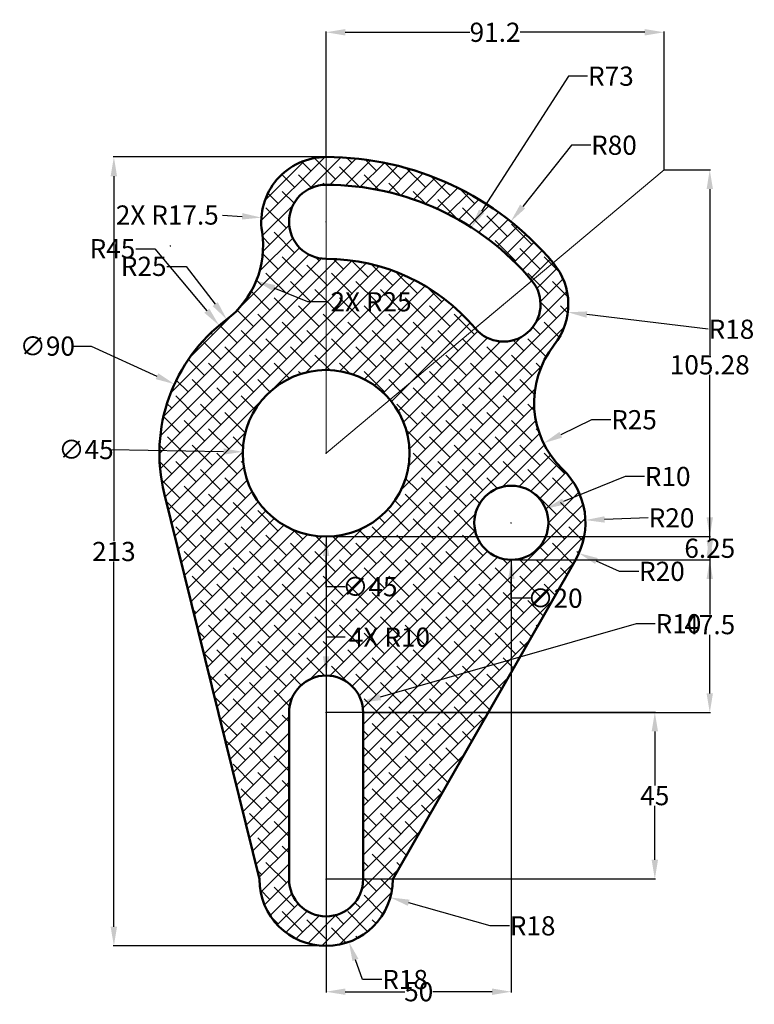
# Model space of a CAD drawing. Units: millimetres. Extents: x 3 to 201, y -134 to 131.
import ezdxf

# ---------------------------------------------------------------- set-up
doc = ezdxf.new("R2010")
doc.units = ezdxf.units.MM
doc.header["$MEASUREMENT"] = 0
for name, color, linetype, lineweight in [('M-CONS', 51, 'Continuous', 13), ('M-DIMS', 85, 'Continuous', 25), ('M-HATC', 241, 'Continuous', 18), ('M-OUTL', 11, 'Continuous', 50)]:
    doc.layers.add(name, color=color, linetype=linetype, lineweight=lineweight)
doc.styles.get("Standard").update_dxf_attribs({"font": 'arial.ttf'})
doc.dimstyles.get("Standard").update_dxf_attribs({"dimtxt": 5.18, "dimasz": 5.18, "dimexe": 0.18, "dimexo": 0.0625, "dimgap": 0.09, "dimtad": 0, "dimtih": 1, "dimtoh": 1, "dimdec": 0, "dimzin": 0, "dimdsep": 46, "dimtxsty": 'Standard', "dimcen": 0.09, "dimadec": 0, "dimazin": 0, "dimtfac": 1, "dimtdec": 0, "dimtofl": 0, "dimtmove": 0, "dimatfit": 3, "dimfxl": 1, "dimtolj": 1, "dimtzin": 0, "dimarcsym": 0})

# ---------------------------------------------------------------- blocks, each defined once
blk = doc.blocks.new('*D1')
at = {"layer": 'Defpoints', "color": 0, "transparency": 16777216}
for p in [(133.74, 54.52), (151.12, 52.43)]:
    blk.add_point(p, dxfattribs=at)
at = {"layer": 'M-DIMS', "color": 0, "lineweight": -2, "transparency": 16777216}
for p, q in [((133.65, 54.52), (133.83, 54.52)), ((133.74, 54.43), (133.74, 54.61)), ((188.99, 47.85), (156.26, 51.8))]:
    blk.add_line(p, q, dxfattribs=at)
at = {"layer": 'M-DIMS', "color": 0, "transparency": 16777216}
blk.add_solid([(156.36, 52.66), (156.15, 50.95), (151.12, 52.43)], dxfattribs=at)
at = {"layer": 'M-DIMS', "color": 0, "transparency": 16777216, "insert": (195.27, 47.85), "char_height": 5.18, "attachment_point": 5}
blk.add_mtext('\\A1;R18', dxfattribs=at)
blk = doc.blocks.new('*D2')
at = {"layer": 'Defpoints', "color": 0, "transparency": 16777216}
for p in [(135.7, 76.93), (85.86, 14.35)]:
    blk.add_point(p, dxfattribs=at)
at = {"layer": 'M-DIMS', "color": 0, "lineweight": -2, "transparency": 16777216}
for p, q in [((152.11, 97.53), (138.93, 80.98)), ((157.29, 97.53), (152.11, 97.53)), ((85.77, 14.35), (85.95, 14.35)), ((85.86, 14.26), (85.86, 14.44))]:
    blk.add_line(p, q, dxfattribs=at)
at = {"layer": 'M-DIMS', "color": 0, "transparency": 16777216}
blk.add_solid([(138.25, 81.52), (139.6, 80.44), (135.7, 76.93)], dxfattribs=at)
at = {"layer": 'M-DIMS', "color": 0, "transparency": 16777216, "insert": (163.56, 97.53), "char_height": 5.18, "attachment_point": 5}
blk.add_mtext('\\A1;R80', dxfattribs=at)
blk = doc.blocks.new('*D3')
at = {"layer": 'Defpoints', "color": 0, "transparency": 16777216}
for p in [(125.05, 75.35), (85.86, 14.35)]:
    blk.add_point(p, dxfattribs=at)
at = {"layer": 'M-DIMS', "color": 0, "lineweight": -2, "transparency": 16777216}
for p, q in [((151.28, 116.17), (127.85, 79.7)), ((156.46, 116.17), (151.28, 116.17)), ((85.77, 14.35), (85.95, 14.35)), ((85.86, 14.26), (85.86, 14.44))]:
    blk.add_line(p, q, dxfattribs=at)
at = {"layer": 'M-DIMS', "color": 0, "transparency": 16777216}
blk.add_solid([(127.13, 80.17), (128.58, 79.24), (125.05, 75.35)], dxfattribs=at)
at = {"layer": 'M-DIMS', "color": 0, "transparency": 16777216, "insert": (162.74, 116.17), "char_height": 5.18, "attachment_point": 5}
blk.add_mtext('\\A1;R73', dxfattribs=at)
blk = doc.blocks.new('*D4')
at = {"layer": 'Defpoints', "color": 0, "transparency": 16777216}
for p in [(167.01, 28.08), (144.56, 17.09)]:
    blk.add_point(p, dxfattribs=at)
at = {"layer": 'M-DIMS', "color": 0, "lineweight": -2, "transparency": 16777216}
for p, q in [((157.5, 23.42), (149.21, 19.36)), ((162.68, 23.42), (157.5, 23.42))]:
    blk.add_line(p, q, dxfattribs=at)
at = {"layer": 'M-DIMS', "color": 0, "transparency": 16777216}
blk.add_solid([(148.83, 20.14), (149.59, 18.59), (144.56, 17.09)], dxfattribs=at)
at = {"layer": 'M-DIMS', "color": 0, "transparency": 16777216, "insert": (168.98, 23.42), "char_height": 5.18, "attachment_point": 5}
blk.add_mtext('\\A1;R25', dxfattribs=at)
blk = doc.blocks.new('*D5')
at = {"layer": 'Defpoints', "color": 0, "transparency": 16777216}
for p in [(135.86, -4.4), (155.85, -3.68)]:
    blk.add_point(p, dxfattribs=at)
at = {"layer": 'M-DIMS', "color": 0, "lineweight": -2, "transparency": 16777216}
for p, q in [((135.77, -4.4), (135.95, -4.4)), ((135.86, -4.49), (135.86, -4.31)), ((172.83, -3.08), (161.03, -3.5))]:
    blk.add_line(p, q, dxfattribs=at)
at = {"layer": 'M-DIMS', "color": 0, "transparency": 16777216}
blk.add_solid([(161, -2.64), (161.06, -4.36), (155.85, -3.68)], dxfattribs=at)
at = {"layer": 'M-DIMS', "color": 0, "transparency": 16777216, "insert": (179.1, -3.08), "char_height": 5.18, "attachment_point": 5}
blk.add_mtext('\\A1;R20', dxfattribs=at)
blk = doc.blocks.new('*D6')
at = {"layer": 'Defpoints', "color": 0, "transparency": 16777216}
for p in [(145.13, -0.63), (135.86, -4.4)]:
    blk.add_point(p, dxfattribs=at)
at = {"layer": 'M-DIMS', "color": 0, "lineweight": -2, "transparency": 16777216}
for p, q in [((166.61, 8.1), (149.93, 1.32)), ((171.79, 8.1), (166.61, 8.1)), ((135.77, -4.4), (135.95, -4.4)), ((135.86, -4.49), (135.86, -4.31))]:
    blk.add_line(p, q, dxfattribs=at)
at = {"layer": 'M-DIMS', "color": 0, "transparency": 16777216}
blk.add_solid([(149.6, 2.12), (150.25, 0.52), (145.13, -0.63)], dxfattribs=at)
at = {"layer": 'M-DIMS', "color": 0, "transparency": 16777216, "insert": (178.06, 8.1), "char_height": 5.18, "attachment_point": 5}
blk.add_mtext('\\A1;R10', dxfattribs=at)
blk = doc.blocks.new('*D7')
at = {"layer": 'Defpoints', "color": 0, "transparency": 16777216}
for p in [(95.48, -52.89), (85.86, -55.65)]:
    blk.add_point(p, dxfattribs=at)
at = {"layer": 'M-DIMS', "color": 0, "lineweight": -2, "transparency": 16777216}
for p, q in [((169.51, -31.65), (100.45, -51.46)), ((174.69, -31.65), (169.51, -31.65)), ((85.77, -55.65), (85.95, -55.65)), ((85.86, -55.74), (85.86, -55.56))]:
    blk.add_line(p, q, dxfattribs=at)
at = {"layer": 'M-DIMS', "color": 0, "transparency": 16777216}
blk.add_solid([(100.22, -50.63), (100.69, -52.29), (95.48, -52.89)], dxfattribs=at)
at = {"layer": 'M-DIMS', "color": 0, "transparency": 16777216, "insert": (180.96, -31.65), "char_height": 5.18, "attachment_point": 5}
blk.add_mtext('\\A1;R10', dxfattribs=at)
blk = doc.blocks.new('*D8')
at = {"layer": 'Defpoints', "color": 0, "transparency": 16777216}
for p in [(85.86, -100.65), (103.18, -105.56)]:
    blk.add_point(p, dxfattribs=at)
at = {"layer": 'M-DIMS', "color": 0, "lineweight": -2, "transparency": 16777216}
for p, q in [((85.77, -100.65), (85.95, -100.65)), ((85.86, -100.74), (85.86, -100.56)), ((130.15, -113.21), (108.16, -106.98)), ((135.33, -113.21), (130.15, -113.21))]:
    blk.add_line(p, q, dxfattribs=at)
at = {"layer": 'M-DIMS', "color": 0, "transparency": 16777216}
blk.add_solid([(108.4, -106.15), (107.93, -107.81), (103.18, -105.56)], dxfattribs=at)
at = {"layer": 'M-DIMS', "color": 0, "transparency": 16777216, "insert": (141.61, -113.21), "char_height": 5.18, "attachment_point": 5}
blk.add_mtext('\\A1;R18', dxfattribs=at)
blk = doc.blocks.new('*D9')
at = {"layer": 'Defpoints', "color": 0, "transparency": 16777216}
for p in [(43.86, 70.35), (59.07, 50.51)]:
    blk.add_point(p, dxfattribs=at)
at = {"layer": 'M-DIMS', "color": 0, "lineweight": -2, "transparency": 16777216}
for p, q in [((42.92, 64.83), (48.1, 64.83)), ((48.1, 64.83), (55.92, 54.62))]:
    blk.add_line(p, q, dxfattribs=at)
at = {"layer": 'M-DIMS', "color": 0, "transparency": 16777216}
blk.add_solid([(56.61, 55.15), (55.24, 54.1), (59.07, 50.51)], dxfattribs=at)
at = {"layer": 'M-DIMS', "color": 0, "transparency": 16777216, "insert": (36.62, 64.83), "char_height": 5.18, "attachment_point": 5}
blk.add_mtext('\\A1;R25', dxfattribs=at)
blk = doc.blocks.new('*D10')
at = {"layer": 'Defpoints', "color": 0, "transparency": 16777216}
for p in [(44.92, 33.03), (126.81, -4.33)]:
    blk.add_point(p, dxfattribs=at)
at = {"layer": 'M-DIMS', "color": 0, "lineweight": -2, "transparency": 16777216}
for p, q in [((17.23, 43.3), (22.41, 43.3)), ((22.41, 43.3), (40.21, 35.18)), ((85.77, 14.35), (85.95, 14.35)), ((85.86, 14.26), (85.86, 14.44))]:
    blk.add_line(p, q, dxfattribs=at)
at = {"layer": 'M-DIMS', "color": 0, "transparency": 16777216}
blk.add_solid([(40.57, 35.96), (39.85, 34.39), (44.92, 33.03)], dxfattribs=at)
at = {"layer": 'M-DIMS', "color": 0, "transparency": 16777216, "insert": (10.62, 43.3), "char_height": 5.18, "attachment_point": 5}
blk.add_mtext('\\A1;∅90', dxfattribs=at)
blk = doc.blocks.new('*D11')
at = {"layer": 'Defpoints', "color": 0, "transparency": 16777216}
for p in [(63.37, 14.75), (108.36, 13.95)]:
    blk.add_point(p, dxfattribs=at)
at = {"layer": 'M-DIMS', "color": 0, "lineweight": -2, "transparency": 16777216}
for p, q in [((27.7, 15.38), (58.19, 14.84)), ((85.77, 14.35), (85.95, 14.35)), ((85.86, 14.26), (85.86, 14.44))]:
    blk.add_line(p, q, dxfattribs=at)
at = {"layer": 'M-DIMS', "color": 0, "transparency": 16777216}
blk.add_solid([(58.2, 15.7), (58.17, 13.98), (63.37, 14.75)], dxfattribs=at)
at = {"layer": 'M-DIMS', "color": 0, "transparency": 16777216, "insert": (21.06, 15.38), "char_height": 5.18, "attachment_point": 5}
blk.add_mtext('\\A1;∅45', dxfattribs=at)
blk = doc.blocks.new('*D12')
at = {"layer": 'Defpoints', "color": 0, "transparency": 16777216}
for p in [(85.86, -55.56), (85.86, -100.56), (174.59, -100.56)]:
    blk.add_point(p, dxfattribs=at)
at = {"layer": 'M-DIMS', "color": 0, "lineweight": -2, "transparency": 16777216}
for p, q in [((85.93, -55.56), (174.77, -55.56)), ((174.59, -60.74), (174.59, -75.34)), ((174.59, -95.38), (174.59, -80.78)), ((85.93, -100.56), (174.77, -100.56))]:
    blk.add_line(p, q, dxfattribs=at)
at = {"layer": 'M-DIMS', "color": 0, "transparency": 16777216}
for points in [[(173.73, -60.74), (175.45, -60.74), (174.59, -55.56)], [(173.73, -95.38), (175.45, -95.38), (174.59, -100.56)]]:
    blk.add_solid(points, dxfattribs=at)
at = {"layer": 'M-DIMS', "color": 0, "transparency": 16777216, "insert": (174.59, -78.06), "char_height": 5.18, "attachment_point": 5}
blk.add_mtext('\\A1;45', dxfattribs=at)
blk = doc.blocks.new('*D13')
at = {"layer": 'Defpoints', "color": 0, "transparency": 16777216}
for p in [(28.58, 94.35), (85.86, 94.35), (85.86, -118.65)]:
    blk.add_point(p, dxfattribs=at)
at = {"layer": 'M-DIMS', "color": 0, "lineweight": -2, "transparency": 16777216}
for p, q in [((85.8, 94.35), (28.4, 94.35)), ((28.58, 89.17), (28.58, -9.41)), ((28.58, -113.47), (28.58, -14.89)), ((85.8, -118.65), (28.4, -118.65))]:
    blk.add_line(p, q, dxfattribs=at)
at = {"layer": 'M-DIMS', "color": 0, "transparency": 16777216}
for points in [[(27.71, 89.17), (29.44, 89.17), (28.58, 94.35)], [(27.71, -113.47), (29.44, -113.47), (28.58, -118.65)]]:
    blk.add_solid(points, dxfattribs=at)
at = {"layer": 'M-DIMS', "color": 0, "transparency": 16777216, "insert": (28.58, -12.15), "char_height": 5.18, "attachment_point": 5}
blk.add_mtext('\\A1;213', dxfattribs=at)
blk = doc.blocks.new('*D14')
at = {"layer": 'Defpoints', "color": 0, "transparency": 16777216}
for p in [(85.86, -8.15), (189.42, -8.15), (95.86, -55.65)]:
    blk.add_point(p, dxfattribs=at)
at = {"layer": 'M-DIMS', "color": 0, "lineweight": -2, "transparency": 16777216}
for p, q in [((85.93, -8.15), (189.6, -8.15)), ((189.42, -13.33), (189.42, -29.18)), ((189.42, -50.47), (189.42, -34.62)), ((95.93, -55.65), (189.6, -55.65))]:
    blk.add_line(p, q, dxfattribs=at)
at = {"layer": 'M-DIMS', "color": 0, "transparency": 16777216}
for points in [[(188.56, -13.33), (190.28, -13.33), (189.42, -8.15)], [(188.56, -50.47), (190.28, -50.47), (189.42, -55.65)]]:
    blk.add_solid(points, dxfattribs=at)
at = {"layer": 'M-DIMS', "color": 0, "transparency": 16777216, "insert": (189.42, -31.9), "char_height": 5.18, "attachment_point": 5}
blk.add_mtext('\\A1;47.5', dxfattribs=at)
blk = doc.blocks.new('*D15')
at = {"layer": 'Defpoints', "color": 0, "transparency": 16777216}
for p in [(85.86, -8.15), (135.86, -14.4), (85.86, -131)]:
    blk.add_point(p, dxfattribs=at)
at = {"layer": 'M-DIMS', "color": 0, "lineweight": -2, "transparency": 16777216}
for p, q in [((85.86, -8.21), (85.86, -131.18)), ((135.86, -14.46), (135.86, -131.18)), ((91.04, -131), (107.07, -131)), ((130.68, -131), (114.65, -131))]:
    blk.add_line(p, q, dxfattribs=at)
at = {"layer": 'M-DIMS', "color": 0, "transparency": 16777216}
for points in [[(91.04, -130.14), (91.04, -131.86), (85.86, -131)], [(130.68, -130.14), (130.68, -131.86), (135.86, -131)]]:
    blk.add_solid(points, dxfattribs=at)
at = {"layer": 'M-DIMS', "color": 0, "transparency": 16777216, "insert": (110.86, -131), "char_height": 5.18, "attachment_point": 5}
blk.add_mtext('\\A1;50', dxfattribs=at)
blk = doc.blocks.new('*D16')
at = {"layer": 'Defpoints', "color": 0, "transparency": 16777216}
for p in [(85.86, -8.15), (189.42, -8.15), (135.86, -14.4)]:
    blk.add_point(p, dxfattribs=at)
at = {"layer": 'M-DIMS', "color": 0, "lineweight": -2, "transparency": 16777216}
for p, q in [((189.42, -2.97), (189.42, 2.21)), ((85.93, -8.15), (189.6, -8.15)), ((135.93, -14.4), (189.6, -14.4)), ((189.42, -19.58), (189.42, -24.76))]:
    blk.add_line(p, q, dxfattribs=at)
at = {"layer": 'M-DIMS', "color": 0, "transparency": 16777216}
for points in [[(188.56, -2.97), (190.28, -2.97), (189.42, -8.15)], [(188.56, -19.58), (190.28, -19.58), (189.42, -14.4)]]:
    blk.add_solid(points, dxfattribs=at)
at = {"layer": 'M-DIMS', "color": 0, "transparency": 16777216, "insert": (189.42, -11.28), "char_height": 5.18, "attachment_point": 5}
blk.add_mtext('\\A1;6.25', dxfattribs=at)
blk = doc.blocks.new('*D17')
at = {"layer": 'Defpoints', "color": 0, "transparency": 16777216}
for p in [(177.07, 128.02), (85.86, 94.35), (177.07, 90.88)]:
    blk.add_point(p, dxfattribs=at)
at = {"layer": 'M-DIMS', "color": 0, "lineweight": -2, "transparency": 16777216}
for p, q in [((85.86, 94.41), (85.86, 128.2)), ((91.04, 128.02), (124.68, 128.02)), ((171.89, 128.02), (138.26, 128.02)), ((177.07, 90.95), (177.07, 128.2))]:
    blk.add_line(p, q, dxfattribs=at)
at = {"layer": 'M-DIMS', "color": 0, "transparency": 16777216}
for points in [[(91.04, 128.88), (91.04, 127.15), (85.86, 128.02)], [(171.89, 128.88), (171.89, 127.15), (177.07, 128.02)]]:
    blk.add_solid(points, dxfattribs=at)
at = {"layer": 'M-DIMS', "color": 0, "transparency": 16777216, "insert": (131.47, 128.02), "char_height": 5.18, "attachment_point": 5}
blk.add_mtext('\\A1;91.2', dxfattribs=at)
blk = doc.blocks.new('*D18')
at = {"layer": 'Defpoints', "color": 0, "transparency": 16777216}
for p in [(177.07, 90.88), (189.42, 90.88), (135.86, -14.4)]:
    blk.add_point(p, dxfattribs=at)
at = {"layer": 'M-DIMS', "color": 0, "lineweight": -2, "transparency": 16777216}
for p, q in [((177.13, 90.88), (189.6, 90.88)), ((189.42, 85.7), (189.42, 40.98)), ((189.42, -9.22), (189.42, 35.51)), ((135.93, -14.4), (189.6, -14.4))]:
    blk.add_line(p, q, dxfattribs=at)
at = {"layer": 'M-DIMS', "color": 0, "transparency": 16777216}
for points in [[(188.56, 85.7), (190.28, 85.7), (189.42, 90.88)], [(188.56, -9.22), (190.28, -9.22), (189.42, -14.4)]]:
    blk.add_solid(points, dxfattribs=at)
at = {"layer": 'M-DIMS', "color": 0, "transparency": 16777216, "insert": (189.42, 38.24), "char_height": 5.18, "attachment_point": 5}
blk.add_mtext('\\A1;105.28', dxfattribs=at)
blk = doc.blocks.new('*D19')
at = {"layer": 'Defpoints', "color": 0, "transparency": 16777216}
for p in [(57, 48.87), (85.86, 14.35)]:
    blk.add_point(p, dxfattribs=at)
at = {"layer": 'M-DIMS', "color": 0, "lineweight": -2, "transparency": 16777216}
for p, q in [((34.5, 69.59), (39.68, 69.59)), ((39.68, 69.59), (53.68, 52.85)), ((85.77, 14.35), (85.95, 14.35)), ((85.86, 14.26), (85.86, 14.44))]:
    blk.add_line(p, q, dxfattribs=at)
at = {"layer": 'M-DIMS', "color": 0, "transparency": 16777216}
blk.add_solid([(54.34, 53.4), (53.01, 52.29), (57, 48.87)], dxfattribs=at)
at = {"layer": 'M-DIMS', "color": 0, "transparency": 16777216, "insert": (28.2, 69.59), "char_height": 5.18, "attachment_point": 5}
blk.add_mtext('\\A1;R45', dxfattribs=at)
blk = doc.blocks.new('*D20')
at = {"layer": 'Defpoints', "color": 0, "transparency": 16777216}
for p in [(43.86, 70.35), (67.02, 60.92)]:
    blk.add_point(p, dxfattribs=at)
at = {"layer": 'M-DIMS', "color": 0, "lineweight": -2, "transparency": 16777216}
for p, q in [((43.77, 70.35), (43.95, 70.35)), ((43.86, 70.26), (43.86, 70.44)), ((80.91, 55.26), (71.81, 58.96)), ((86.09, 55.26), (80.91, 55.26))]:
    blk.add_line(p, q, dxfattribs=at)
at = {"layer": 'M-DIMS', "color": 0, "transparency": 16777216}
blk.add_solid([(72.14, 59.76), (71.49, 58.16), (67.02, 60.92)], dxfattribs=at)
at = {"layer": 'M-DIMS', "color": 0, "transparency": 16777216, "insert": (98, 55.26), "char_height": 5.18, "attachment_point": 5}
blk.add_mtext('\\A1;2X R25', dxfattribs=at)
blk = doc.blocks.new('*D21')
at = {"layer": 'Defpoints', "color": 0, "transparency": 16777216}
for p in [(85.86, 36.85), (85.86, -8.15)]:
    blk.add_point(p, dxfattribs=at)
at = {"layer": 'M-DIMS', "color": 0, "lineweight": -2, "transparency": 16777216}
for p, q in [((85.77, 14.35), (85.95, 14.35)), ((85.86, 14.26), (85.86, 14.44)), ((85.86, -21.65), (85.86, -13.33)), ((91.04, -21.65), (85.86, -21.65))]:
    blk.add_line(p, q, dxfattribs=at)
at = {"layer": 'M-DIMS', "color": 0, "transparency": 16777216}
blk.add_solid([(86.73, -13.33), (85, -13.33), (85.86, -8.15)], dxfattribs=at)
at = {"layer": 'M-DIMS', "color": 0, "transparency": 16777216, "insert": (97.68, -21.65), "char_height": 5.18, "attachment_point": 5}
blk.add_mtext('\\A1;∅45', dxfattribs=at)
blk = doc.blocks.new('*D22')
at = {"layer": 'Defpoints', "color": 0, "transparency": 16777216}
for p in [(135.86, -4.4), (154.11, -12.6)]:
    blk.add_point(p, dxfattribs=at)
at = {"layer": 'M-DIMS', "color": 0, "lineweight": -2, "transparency": 16777216}
for p, q in [((135.77, -4.4), (135.95, -4.4)), ((135.86, -4.49), (135.86, -4.31)), ((165.05, -17.51), (158.83, -14.72)), ((170.23, -17.51), (165.05, -17.51))]:
    blk.add_line(p, q, dxfattribs=at)
at = {"layer": 'M-DIMS', "color": 0, "transparency": 16777216}
blk.add_solid([(159.19, -13.93), (158.48, -15.51), (154.11, -12.6)], dxfattribs=at)
at = {"layer": 'M-DIMS', "color": 0, "transparency": 16777216, "insert": (176.5, -17.51), "char_height": 5.18, "attachment_point": 5}
blk.add_mtext('\\A1;R20', dxfattribs=at)
blk = doc.blocks.new('*D23')
at = {"layer": 'Defpoints', "color": 0, "transparency": 16777216}
for p in [(85.86, -100.65), (92.02, -117.56)]:
    blk.add_point(p, dxfattribs=at)
at = {"layer": 'M-DIMS', "color": 0, "lineweight": -2, "transparency": 16777216}
for p, q in [((85.77, -100.65), (85.95, -100.65)), ((85.86, -100.74), (85.86, -100.56)), ((95.72, -127.71), (93.79, -122.43)), ((100.9, -127.71), (95.72, -127.71))]:
    blk.add_line(p, q, dxfattribs=at)
at = {"layer": 'M-DIMS', "color": 0, "transparency": 16777216}
blk.add_solid([(94.6, -122.14), (92.98, -122.73), (92.02, -117.56)], dxfattribs=at)
at = {"layer": 'M-DIMS', "color": 0, "transparency": 16777216, "insert": (107.18, -127.71), "char_height": 5.18, "attachment_point": 5}
blk.add_mtext('\\A1;R18', dxfattribs=at)
blk = doc.blocks.new('*D24')
at = {"layer": 'Defpoints', "color": 0, "transparency": 16777216}
for p in [(68.4, 77.99), (85.86, 76.85)]:
    blk.add_point(p, dxfattribs=at)
at = {"layer": 'M-DIMS', "color": 0, "lineweight": -2, "transparency": 16777216}
for p, q in [((57.92, 78.68), (63.23, 78.33)), ((85.77, 76.85), (85.95, 76.85)), ((85.86, 76.76), (85.86, 76.94))]:
    blk.add_line(p, q, dxfattribs=at)
at = {"layer": 'M-DIMS', "color": 0, "transparency": 16777216}
blk.add_solid([(63.29, 79.19), (63.18, 77.47), (68.4, 77.99)], dxfattribs=at)
at = {"layer": 'M-DIMS', "color": 0, "transparency": 16777216, "insert": (43, 78.68), "char_height": 5.18, "attachment_point": 5}
blk.add_mtext('\\A1;2X R17.5', dxfattribs=at)
blk = doc.blocks.new('*D25')
at = {"layer": 'Defpoints', "color": 0, "transparency": 16777216}
for p in [(85.86, -45.65), (85.86, -55.65)]:
    blk.add_point(p, dxfattribs=at)
at = {"layer": 'M-DIMS', "color": 0, "lineweight": -2, "transparency": 16777216}
for p, q in [((91.04, -35.29), (85.86, -35.29)), ((85.86, -35.29), (85.86, -40.47)), ((85.77, -55.65), (85.95, -55.65)), ((85.86, -55.74), (85.86, -55.56))]:
    blk.add_line(p, q, dxfattribs=at)
at = {"layer": 'M-DIMS', "color": 0, "transparency": 16777216}
blk.add_solid([(85, -40.47), (86.73, -40.47), (85.86, -45.65)], dxfattribs=at)
at = {"layer": 'M-DIMS', "color": 0, "transparency": 16777216, "insert": (102.98, -35.29), "char_height": 5.18, "attachment_point": 5}
blk.add_mtext('\\A1;4X R10', dxfattribs=at)
blk = doc.blocks.new('*D26')
at = {"layer": 'Defpoints', "color": 0, "transparency": 16777216}
for p in [(135.86, 5.6), (135.86, -14.4)]:
    blk.add_point(p, dxfattribs=at)
at = {"layer": 'M-DIMS', "color": 0, "lineweight": -2, "transparency": 16777216}
for p, q in [((135.77, -4.4), (135.95, -4.4)), ((135.86, -4.49), (135.86, -4.31)), ((135.86, -24.76), (135.86, -19.58)), ((141.04, -24.76), (135.86, -24.76))]:
    blk.add_line(p, q, dxfattribs=at)
at = {"layer": 'M-DIMS', "color": 0, "transparency": 16777216}
blk.add_solid([(136.73, -19.58), (135, -19.58), (135.86, -14.4)], dxfattribs=at)
at = {"layer": 'M-DIMS', "color": 0, "transparency": 16777216, "insert": (147.65, -24.76), "char_height": 5.18, "attachment_point": 5}
blk.add_mtext('\\A1;∅20', dxfattribs=at)

msp = doc.modelspace()

# ---------------------------------------------------------------- hatches: boundary and pattern name
at = {"layer": 'M-HATC'}
h = msp.add_hatch(dxfattribs=at)
h.set_pattern_fill('ANSI38', color=256, scale=25)
h.paths.add_polyline_path([(153.225, -14.328, 0.3441363), (149.707, 10.035, -0.3872696), (147.441, 43.635, 0.3564827), (147.147, 65.773), (141.402, 60.952, -1), (126.081, 48.096), (103.1, 28.813, -0.176327), (108.364, 14.35, -1), (63.364, 14.35, -0.4142136), (85.864, 36.85), (85.864, 66.85, -1), (85.864, 86.85), (85.864, 94.35, 0.4599349), (68.569, 74.173, -0.276984), (58.864, 50.35, 0.3008573), (42.171, 3.58), (67.864, -100.65, 1), (103.864, -100.65)])
h.paths.add_polyline_path([(95.864, -55.65), (95.864, -100.65, -1), (75.864, -100.65), (75.864, -55.65, -1)], flags=16)
h.paths.add_polyline_path([(125.864, -4.4, -1), (145.864, -4.4, -1)], flags=16)
h.paths.add_polyline_path([(85.864, 94.35), (85.864, 86.85, -0.2216947), (141.402, 60.952), (147.147, 65.773, 0.2216947)])
h = msp.add_hatch(dxfattribs=at)
h.set_pattern_fill('ANSI38', color=256, scale=25)
h.paths.add_polyline_path([(126.081, 48.096, 0.2216947), (85.864, 66.85), (85.864, 36.85, -0.2216947), (103.1, 28.813)])

# ---------------------------------------------------------------- linework, layer by layer
at = {"layer": 'M-CONS'}
for p, q in [((85.864, 14.35), (85.864, 115.668)), ((85.864, 14.35), (177.072, 90.883)), ((126.081, 48.096), (141.402, 60.952))]:
    msp.add_line(p, q, dxfattribs=at)
at = {"layer": 'M-OUTL'}
for p, q in [((67.864, -100.65), (42.171, 3.58)), ((103.864, -100.65), (153.225, -14.328)), ((75.864, -55.65), (75.864, -100.65)), ((95.864, -55.65), (95.864, -100.65))]:
    msp.add_line(p, q, dxfattribs=at)
for centre, radius in [((85.864, 14.35), 22.5), ((135.864, -4.4), 10)]:
    msp.add_circle(centre, radius, dxfattribs=at)
for centre, radius, start, end in [((85.864, 76.85), 17.5, 90, 188.79741), ((85.864, 14.35), 80, 40, 90), ((85.864, 76.85), 10, 90, 270), ((85.864, 14.35), 72.5, 40, 90), ((43.864, 70.35), 25, 306.8699, 8.79741), ((85.864, 14.35), 52.5, 40, 90), ((133.741, 54.524), 17.5, 321.51891, 40), ((133.741, 54.524), 10, 220, 40), ((85.864, 14.35), 45, 126.8699, 193.84709), ((167.011, 28.078), 25, 141.51891, 226.19839), ((135.864, -4.4), 20, 330.2376, 46.19839), ((85.864, -55.65), 10, 0, 180), ((85.864, -100.65), 18, 180, 360), ((85.864, -100.65), 10, 180, 0)]:
    msp.add_arc(centre, radius, start, end, dxfattribs=at)

# ---------------------------------------------------------------- dimensions: what is measured, and where the dimension line sits
at = {"layer": 'M-DIMS'}
for base, p1, p2, override, picture, middle in [((177.072, 128.018), (85.864, 94.35), (177.072, 90.883), {"dimdec": 1, "dimlfac": 1, "dimrnd": 0, "dimzin": 0, "dimdsep": 46, "dimlunit": 2}, '*D17', (131.468, 128.018)), ((85.864, -131), (135.864, -14.4), (85.864, -8.15), {"dimdec": 0, "dimlfac": 1, "dimrnd": 0, "dimzin": 0, "dimdsep": 46, "dimlunit": 2}, '*D15', (110.864, -131))]:
    dim = msp.add_linear_dim(base=base, p1=p1, p2=p2, dimstyle='Standard', override=override, dxfattribs=at)
    dim.commit()
    dim.dimension.update_dxf_attribs({"geometry": picture, "text_midpoint": middle})
for center, mpoint, override, picture, middle in [((85.8636, 14.3499), (125.0534, 75.3451), {"dimclrd": 0, "dimclre": 0, "dimclrt": 0}, '*D3', (162.7402, 116.1666)), ((85.864, 14.35), (135.701, 76.93), {"dimclrd": 0, "dimclre": 0, "dimclrt": 0}, '*D2', (163.56, 97.535)), ((85.864, 14.35), (56.998, 48.872), {"dimdec": 0, "dimlfac": 1, "dimrnd": 0, "dimzin": 0, "dimdsep": 46, "dimlunit": 2}, '*D19', (28.201, 69.586)), ((43.864, 70.35), (59.074, 50.509), {"dimclrd": 0, "dimclre": 0, "dimclrt": 0}, '*D9', (36.62, 64.826)), ((133.741, 54.524), (151.115, 52.425), {"dimclrd": 0, "dimclre": 0, "dimclrt": 0}, '*D1', (188.991, 47.85)), ((167.011, 28.078), (144.557, 17.087), {"dimclrd": 0, "dimclre": 0, "dimclrt": 0}, '*D4', (168.976, 23.422)), ((135.864, -4.4), (145.127, -0.634), {"dimclrd": 0, "dimclre": 0, "dimclrt": 0}, '*D6', (178.064, 8.102)), ((135.864, -4.4), (155.851, -3.685), {"dimclrd": 0, "dimclre": 0, "dimclrt": 0}, '*D5', (172.83, -3.077)), ((135.864, -4.4), (154.107, -12.597), {"dimdec": 0, "dimlfac": 1, "dimrnd": 0, "dimzin": 0, "dimdsep": 46, "dimlunit": 2}, '*D22', (176.503, -17.515)), ((85.864, -55.65), (95.476, -52.892), {"dimclrd": 0, "dimclre": 0, "dimclrt": 0}, '*D7', (180.965, -31.646)), ((85.864, -100.65), (103.18, -105.562), {"dimclrd": 0, "dimclre": 0, "dimclrt": 0}, '*D8', (141.612, -113.212)), ((85.864, -100.65), (92.021, -117.564), {"dimdec": 0, "dimlfac": 1, "dimrnd": 0, "dimzin": 0, "dimdsep": 46, "dimlunit": 2}, '*D23', (107.18, -127.712))]:
    dim = msp.add_radius_dim(center=center, mpoint=mpoint, dimstyle='Standard', override=override, dxfattribs=at)
    dim.commit()
    dim.dimension.update_dxf_attribs({"geometry": picture, "text_midpoint": middle, "dimtype": 164})
for base, p1, p2, override, picture, middle in [((28.576, 94.35), (85.864, -118.65), (85.864, 94.35), {"dimdec": 0, "dimlfac": 1, "dimrnd": 0, "dimzin": 0, "dimdsep": 46, "dimlunit": 2}, '*D13', (28.576, -12.15)), ((189.422, 90.883), (135.864, -14.4), (177.072, 90.883), {"dimdec": 2, "dimlfac": 1, "dimrnd": 0, "dimzin": 0, "dimdsep": 46, "dimlunit": 2}, '*D18', (189.422, 38.241)), ((189.422, -8.15), (135.864, -14.4), (85.864, -8.15), {"dimdec": 2, "dimlfac": 1, "dimrnd": 0, "dimzin": 0, "dimdsep": 46, "dimlunit": 2}, '*D16', (189.422, -11.275)), ((189.422, -8.15), (95.864, -55.65), (85.864, -8.15), {"dimdec": 1, "dimlfac": 1, "dimrnd": 0, "dimzin": 0, "dimdsep": 46, "dimlunit": 2}, '*D14', (189.422, -31.9))]:
    dim = msp.add_linear_dim(base=base, p1=p1, p2=p2, angle=90, dimstyle='Standard', override=override, dxfattribs=at)
    dim.commit()
    dim.dimension.update_dxf_attribs({"geometry": picture, "text_midpoint": middle})
for center, mpoint, override, picture, middle in [((85.864, 76.85), (68.401, 77.993), {"dimdec": 1, "dimlfac": 1, "dimrnd": 0, "dimzin": 0, "dimdsep": 46, "dimlunit": 2}, '*D24', (57.923, 78.679)), ((43.864, 70.35), (67.016, 60.918), {"dimdec": 0, "dimlfac": 1, "dimrnd": 0, "dimzin": 0, "dimdsep": 46, "dimlunit": 2}, '*D20', (97.995, 55.259))]:
    dim = msp.add_radius_dim(center=center, mpoint=mpoint, text='2X <>', dimstyle='Standard', override=override, dxfattribs=at)
    dim.commit()
    dim.dimension.update_dxf_attribs({"geometry": picture, "text_midpoint": middle, "dimtype": 164})
for p1, p2, override, picture, middle in [((126.805, -4.325), (44.922, 33.025), {"dimclrd": 0, "dimclre": 0, "dimclrt": 0}, '*D10', (10.617, 43.296)), ((85.863, 36.85), (85.864, -8.15), {"dimdec": 0, "dimlfac": 1, "dimrnd": 0, "dimzin": 0, "dimdsep": 46, "dimlunit": 2}, '*D21', (97.682, -21.65)), ((108.36, 13.951), (63.367, 14.749), {"dimclrd": 0, "dimclre": 0, "dimclrt": 0}, '*D11', (27.697, 15.381)), ((135.863, 5.6), (135.864, -14.4), {"dimdec": 0, "dimlfac": 1, "dimrnd": 0, "dimzin": 0, "dimdsep": 46, "dimlunit": 2}, '*D26', (147.654, -24.76))]:
    dim = msp.add_diameter_dim_2p(p1=p1, p2=p2, dimstyle='Standard', override=override, dxfattribs=at)
    dim.commit()
    dim.dimension.update_dxf_attribs({"geometry": picture, "text_midpoint": middle, "dimtype": 163})
dim = msp.add_radius_dim(center=(85.864, -55.65), mpoint=(85.864, -45.65), text='4X <>', dimstyle='Standard', override={"dimdec": 0, "dimlfac": 1, "dimrnd": 0, "dimzin": 0, "dimdsep": 46, "dimlunit": 2}, dxfattribs=at)
dim.commit()
dim.dimension.update_dxf_attribs({"geometry": '*D25', "text_midpoint": (102.984, -35.29)})
dim = msp.add_aligned_dim(p1=(85.864, -55.56), p2=(85.864, -100.56), distance=88.727, dimstyle='Standard', override={"dimclrd": 0, "dimclre": 0, "dimclrt": 0}, dxfattribs=at)
dim.commit()
dim.dimension.update_dxf_attribs({"geometry": '*D12', "text_midpoint": (174.591, -78.06)})

doc.saveas('drawing.dxf')
